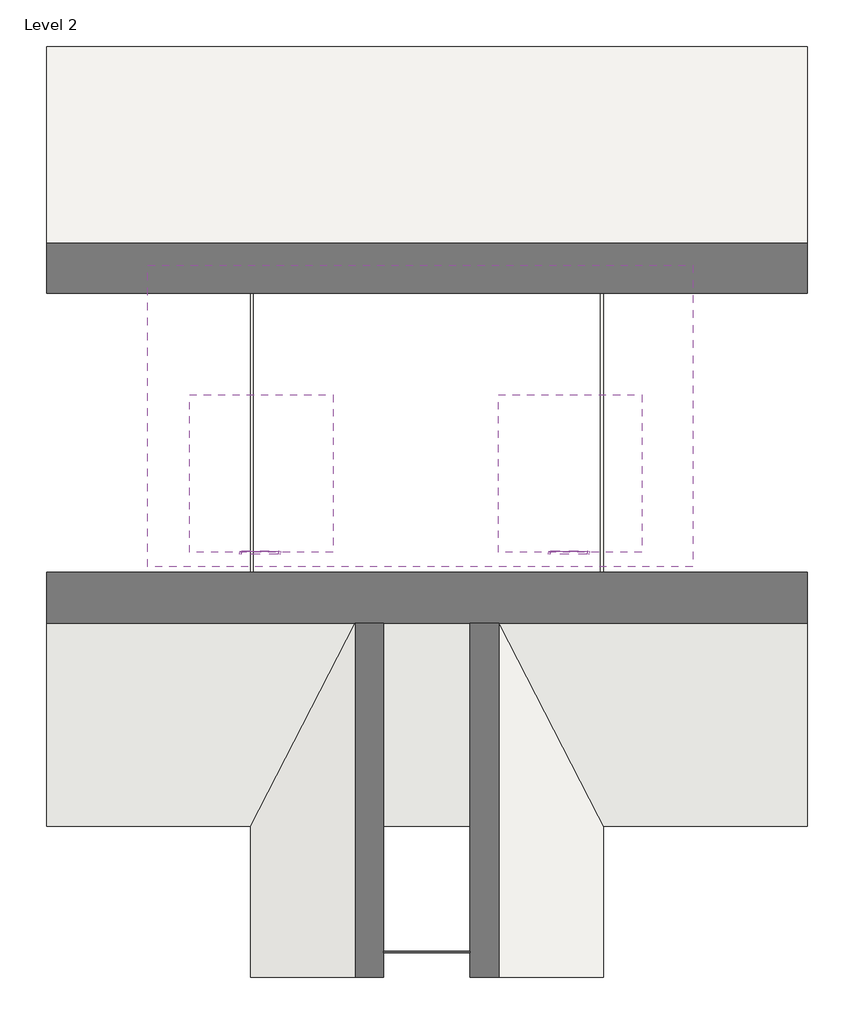
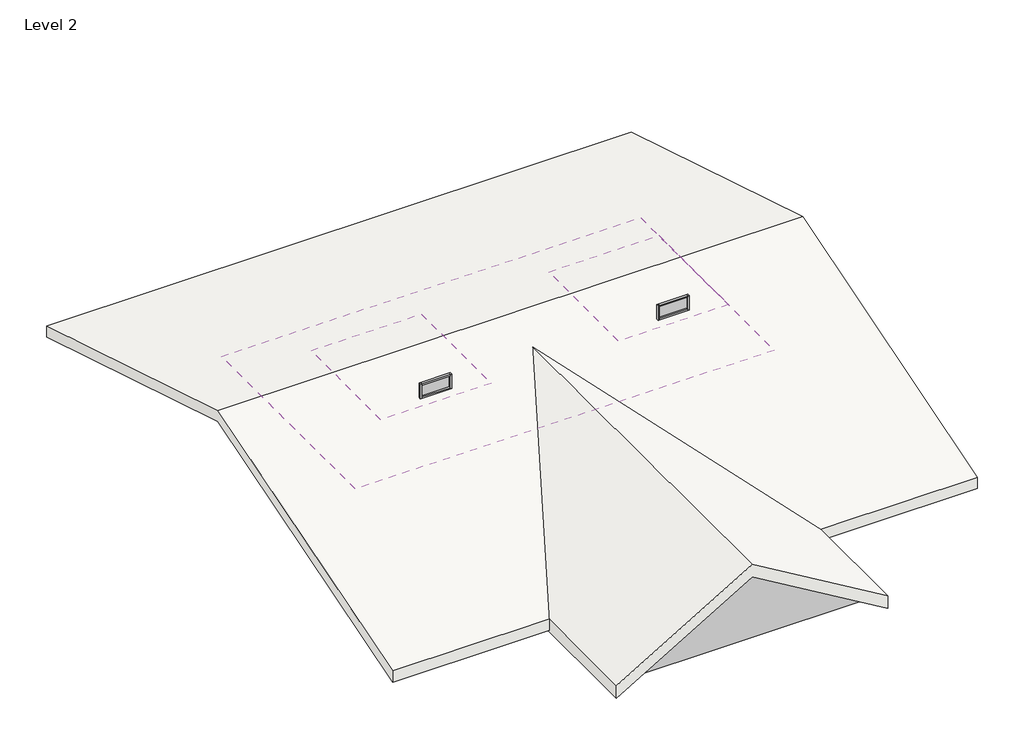
# One storey: 8 members, 5 roofs, 3 plates.
"""IFC4 building model written with IfcOpenShell, lengths in millimetres."""

from ifc_helpers import new_model, si_unit, frame, origin, place, context, project, spatial, polyline, outline, extrude, faceted_brep, transform, mapped, element, save
from components import member_1d97dc70, member_5c5532da, system_panel_glazed_4284b2b2, system_panel_glazed_4f752865

model = new_model("IFC4")

# Units and contexts
model_context = context("Model", 3, world=origin())
ifc_project = project(units=[si_unit("LENGTHUNIT", "METRE", prefix="MILLI")], contexts=[model_context])

# Site, building, storey
site = spatial("IfcSite", under=ifc_project)
building = spatial("IfcBuilding", under=site)
storey = spatial("IfcBuildingStorey", under=building, Name="Level 2", Elevation=3657.6)

# Members
placement = place(None, origin())
member_shape = member_1d97dc70(model_context)
element("IfcMember", 1, ObjectType="Rectangular Mullion : 1.5\" x 2.5\" rectangular", at=placement, inside=storey, context=model_context, shape_type="MappedRepresentation", body=[
    mapped(member_shape, transform((-3966.4771146, 3696.4942616, 6915.4949064), x_axis=(0.0, 0.0, 1.0), y_axis=(0.0, -1.0, 0.0), z_axis=(1.0, 0.0, 0.0))),
])
element("IfcMember", 2, ObjectType="Rectangular Mullion : 1.5\" x 2.5\" rectangular", at=placement, inside=storey, context=model_context, shape_type="MappedRepresentation", body=[
    mapped(member_shape, transform((2408.6929711, 3696.4942616, 6915.4949064), x_axis=(0.0, 0.0, 1.0), y_axis=(0.0, -1.0, 0.0), z_axis=(1.0, 0.0, 0.0))),
])
element("IfcMember", 3, ObjectType="Rectangular Mullion : 1.5\" x 2.5\" rectangular", at=placement, inside=storey, context=model_context, shape_type="MappedRepresentation", body=[
    mapped(member_shape, transform((-4728.4771146, 3696.4942616, 6502.2771866), x_axis=(0.0, 0.0, -1.0), y_axis=(0.0, -1.0, 0.0), z_axis=(-1.0, 0.0, 0.0))),
])
element("IfcMember", 4, ObjectType="Rectangular Mullion : 1.5\" x 2.5\" rectangular", at=placement, inside=storey, context=model_context, shape_type="MappedRepresentation", body=[
    mapped(member_shape, transform((1646.6929711, 3696.4942616, 6502.2771866), x_axis=(0.0, 0.0, -1.0), y_axis=(0.0, -1.0, 0.0), z_axis=(-1.0, 0.0, 0.0))),
])
member_2_shape = member_5c5532da(model_context)
element("IfcMember", 5, ObjectType="Rectangular Mullion : 1.5\" x 2.5\" rectangular", at=placement, inside=storey, context=model_context, shape_type="MappedRepresentation", body=[
    mapped(member_2_shape, transform((-4766.5771146, 3696.4942616, 6915.4949064), x_axis=(-1.0, 0.0, 0.0), y_axis=(0.0, -1.0, 0.0), z_axis=(0.0, 0.0, 1.0))),
])
element("IfcMember", 6, ObjectType="Rectangular Mullion : 1.5\" x 2.5\" rectangular", at=placement, inside=storey, context=model_context, shape_type="MappedRepresentation", body=[
    mapped(member_2_shape, transform((1608.5929711, 3696.4942616, 6915.4949064), x_axis=(-1.0, 0.0, 0.0), y_axis=(0.0, -1.0, 0.0), z_axis=(0.0, 0.0, 1.0))),
])
element("IfcMember", 7, ObjectType="Rectangular Mullion : 1.5\" x 2.5\" rectangular", at=placement, inside=storey, context=model_context, shape_type="MappedRepresentation", body=[
    mapped(member_2_shape, transform((-3928.3771146, 3696.4942616, 6502.2771866), x_axis=(1.0, 0.0, 0.0), y_axis=(0.0, -1.0, 0.0), z_axis=(0.0, 0.0, -1.0))),
])
element("IfcMember", 8, ObjectType="Rectangular Mullion : 1.5\" x 2.5\" rectangular", at=placement, inside=storey, context=model_context, shape_type="MappedRepresentation", body=[
    mapped(member_2_shape, transform((2446.7929711, 3696.4942616, 6502.2771866), x_axis=(1.0, 0.0, 0.0), y_axis=(0.0, -1.0, 0.0), z_axis=(0.0, 0.0, -1.0))),
])

# Plates
system_panel_glazed_shape = system_panel_glazed_4284b2b2(model_context)
element("IfcPlate", 9, ObjectType="System Panel : Glazed", at=placement, inside=storey, context=model_context, shape_type="MappedRepresentation", body=[
    mapped(system_panel_glazed_shape, transform((-905.7652342, -4567.2440778, 3258.0663849), x_axis=(1.0, 0.0, 0.0), y_axis=(0.0, 1.0, 0.0), z_axis=(0.0, 0.0, 1.0))),
])
system_panel_glazed_2_shape = system_panel_glazed_4f752865(model_context)
element("IfcPlate", 10, ObjectType="System Panel : Glazed", at=placement, inside=storey, context=model_context, shape_type="MappedRepresentation", body=[
    mapped(system_panel_glazed_2_shape, transform((-4347.4771146, 3696.4942616, 6540.3771866), x_axis=(1.0, 0.0, 0.0), y_axis=(0.0, 1.0, 0.0), z_axis=(0.0, 0.0, 1.0))),
])
element("IfcPlate", 11, ObjectType="System Panel : Glazed", at=placement, inside=storey, context=model_context, shape_type="MappedRepresentation", body=[
    mapped(system_panel_glazed_2_shape, transform((2027.6929711, 3696.4942616, 6540.3771866), x_axis=(1.0, 0.0, 0.0), y_axis=(0.0, 1.0, 0.0), z_axis=(0.0, 0.0, 1.0))),
])

# Roofs
element("IfcRoof", 12, ObjectType="Generic - 12\"", at=placement, inside=storey, context=model_context, shape_type="SweptSolid", body=[
    extrude(outline(polyline([(14138.6067493, 3621.3506801), (14138.6067493, 3302.6238327), (6171.4405664, 5738.4309791), (-1941.4664613, 3258.0663849), (-1941.4664613, 3576.7932323), (6171.4405664, 6057.1578265), (14138.6067493, 3621.3506801)])), frame((-8754.3652342, 0.0, 0.0), z_axis=(1.0, 0.0, 0.0), x_axis=(0.0, 1.0, 0.0)), (0.0, 0.0, 1.0), 15697.2),
])
element("IfcRoof", 13, ObjectType="Generic - 12\"", at=placement, inside=storey, context=model_context, shape_type="Brep", body=[
    faceted_brep([(-4546.0914635, -5062.5371224, 3576.7932323), (-4546.0914635, -5062.5371224, 3222.2222569), (-905.7652342, -5062.5371224, 5385.8290246), (2734.5609951, -5062.5371224, 3222.2222569), (2734.5609951, -5062.5371224, 3576.7932323), (-905.7652342, -5062.5371224, 5740.4), (-905.7652342, 5135.3724002, 5740.4), (-4546.0914635, -1941.4664613, 3576.7932323), (2734.5609951, -1941.4664613, 3576.7932323), (2734.5609951, 14020.0405664, 3222.2222569), (2734.5609951, 14020.0405664, 3258.0663849), (2734.5609951, -1941.4664613, 3258.0663849), (-905.7652342, 3975.6229969, 5385.8290246), (2137.9858498, -1941.4664613, 3576.7932323), (2674.2522915, -1941.4664613, 3258.0663849), (2674.2522915, 14020.0405664, 3258.0663849), (-4546.0914635, 14020.0405664, 3222.2222569), (-4485.7827599, 14020.0405664, 3258.0663849), (-4485.7827599, -1941.4664613, 3258.0663849), (-3949.5163182, -1941.4664613, 3576.7932323), (-4546.0914635, -1941.4664613, 3258.0663849), (-4546.0914635, 14020.0405664, 3258.0663849)], [[[0, 1, 2, 3, 4, 5]], [[6, 7, 0, 5]], [[8, 6, 5, 4]], [[9, 10, 11, 8, 4, 3]], [[12, 13, 14, 15, 9, 3, 2]], [[16, 17, 18, 19, 12, 2, 1]], [[7, 20, 21, 16, 1, 0]], [[17, 16, 21]], [[10, 9, 15]], [[20, 18, 17, 21]], [[14, 11, 10, 15]], [[7, 6, 8, 13, 12, 19]], [[8, 11, 14, 13]], [[19, 18, 20, 7]]]),
])
element("IfcRoof", 14, ObjectType="Generic - 12\"", at=placement, inside=storey, context=model_context, shape_type="SweptSolid", body=[
    extrude(outline(polyline([(3412.0664332, 5740.4), (6213.5422584, 7702.0144909), (9628.5840845, 5143.4044843), (9628.5840845, 4762.5474916), (6207.4951043, 7325.6881334), (3412.0664332, 5368.3079053), (3412.0664332, 5740.4)])), frame((-6665.2152342, 0.0, 0.0), z_axis=(1.0, 0.0, 0.0), x_axis=(0.0, 1.0, 0.0)), (0.0, 0.0, 1.0), 11245.85),
])
element("IfcRoof", 15, ObjectType="Generic - 12\"", at=placement, inside=storey, context=model_context, shape_type="SweptSolid", body=[
    extrude(outline(polyline([(6669.4367958, -2844.899332), (8079.541847, -4324.604279), (6669.4367958, -5804.309226), (6248.4, -5804.309226), (7658.5050511, -4324.604279), (6248.4, -2844.899332), (6669.4367958, -2844.899332)])), frame((0.0, 3707.6405664, 0.0), z_axis=(0.0, 1.0, 0.0), x_axis=(0.0, 0.0, 1.0)), (0.0, 0.0, 1.0), 3245.934684),
])
element("IfcRoof", 16, ObjectType="Generic - 12\"", at=placement, inside=storey, context=model_context, shape_type="SweptSolid", body=[
    extrude(outline(polyline([(6669.4367958, 3530.2707538), (8079.541847, 2050.5658068), (6669.4367958, 570.8608598), (6248.4, 570.8608598), (7658.5050511, 2050.5658068), (6248.4, 3530.2707538), (6669.4367958, 3530.2707538)])), frame((0.0, 3707.6405664, 0.0), z_axis=(0.0, 1.0, 0.0), x_axis=(0.0, 0.0, 1.0)), (0.0, 0.0, 1.0), 3245.934684),
])

save(model, "model.ifc")

# Revit data of these elements
# Type "Rectangular Mullion : 1.5\" x 2.5\" rectangular"
#   built-in parameter 1007304 = 0.208333 (stored number, unit not read)
#   built-in parameter 1007301 = 0.0625 (stored number, unit not read)
#   built-in parameter 1007300 = 0.0625 (stored number, unit not read)
# Type "System Panel : Glazed"
#   Construction Type Id = "GSP4R"
#   Analytic Construction = "1/8 in Pilkington single glazing"
#   Visual Light Transmittance = 0.9
#   Solar Heat Gain Coefficient = 0.86
#   Heat Transfer Coefficient (U) = 1.18115 BTU/(h·ft²·°F)
#   Define Thermal Properties by = 1
# Type "Generic - 12\""
#   Assembly Code = "B1020"
# Elements 1, 2, 3, 4, 5, 6, 7, 8 (IfcMember, "Rectangular Mullion : 1.5\" x 2.5\" rectangular")
#   Phase Created = New Construction
# Elements 9, 10, 11 (IfcPlate, "System Panel : Glazed")
#   Phase Created = New Construction
#   Materials on its faces: "Glass"
# Elements 12, 13, 14 (IfcRoof, "Generic - 12\"")
#   built-in parameter 1001710 = 33615
#   Phase Created = New Construction
# Elements 15, 16 (IfcRoof, "Generic - 12\"")
#   built-in parameter 1001705 = 26.5077 (stored number, unit not read)
#   built-in parameter 1001701 = 8.5 (stored number, unit not read)
#   built-in parameter 1001710 = 33615
#   Phase Created = New Construction
# Materials
#   "Glass": class "Glass", colour RGB 0 128 192, transparency 0.75, Description = "Soda Lime Glass", Cost = 0
